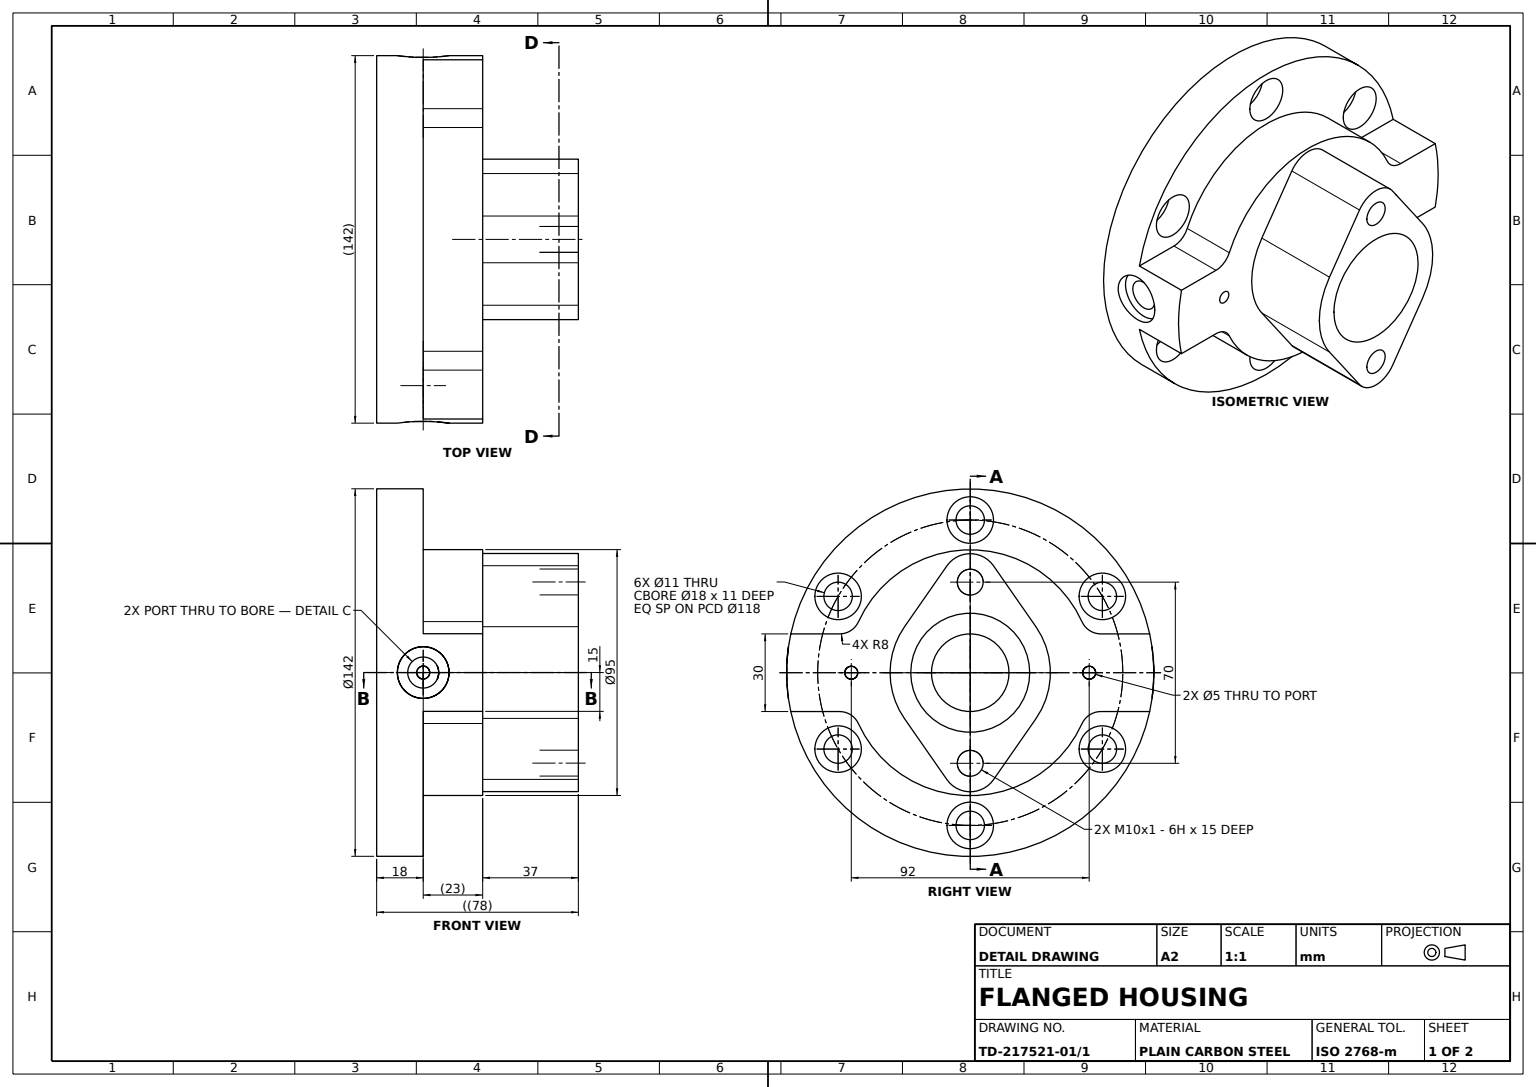
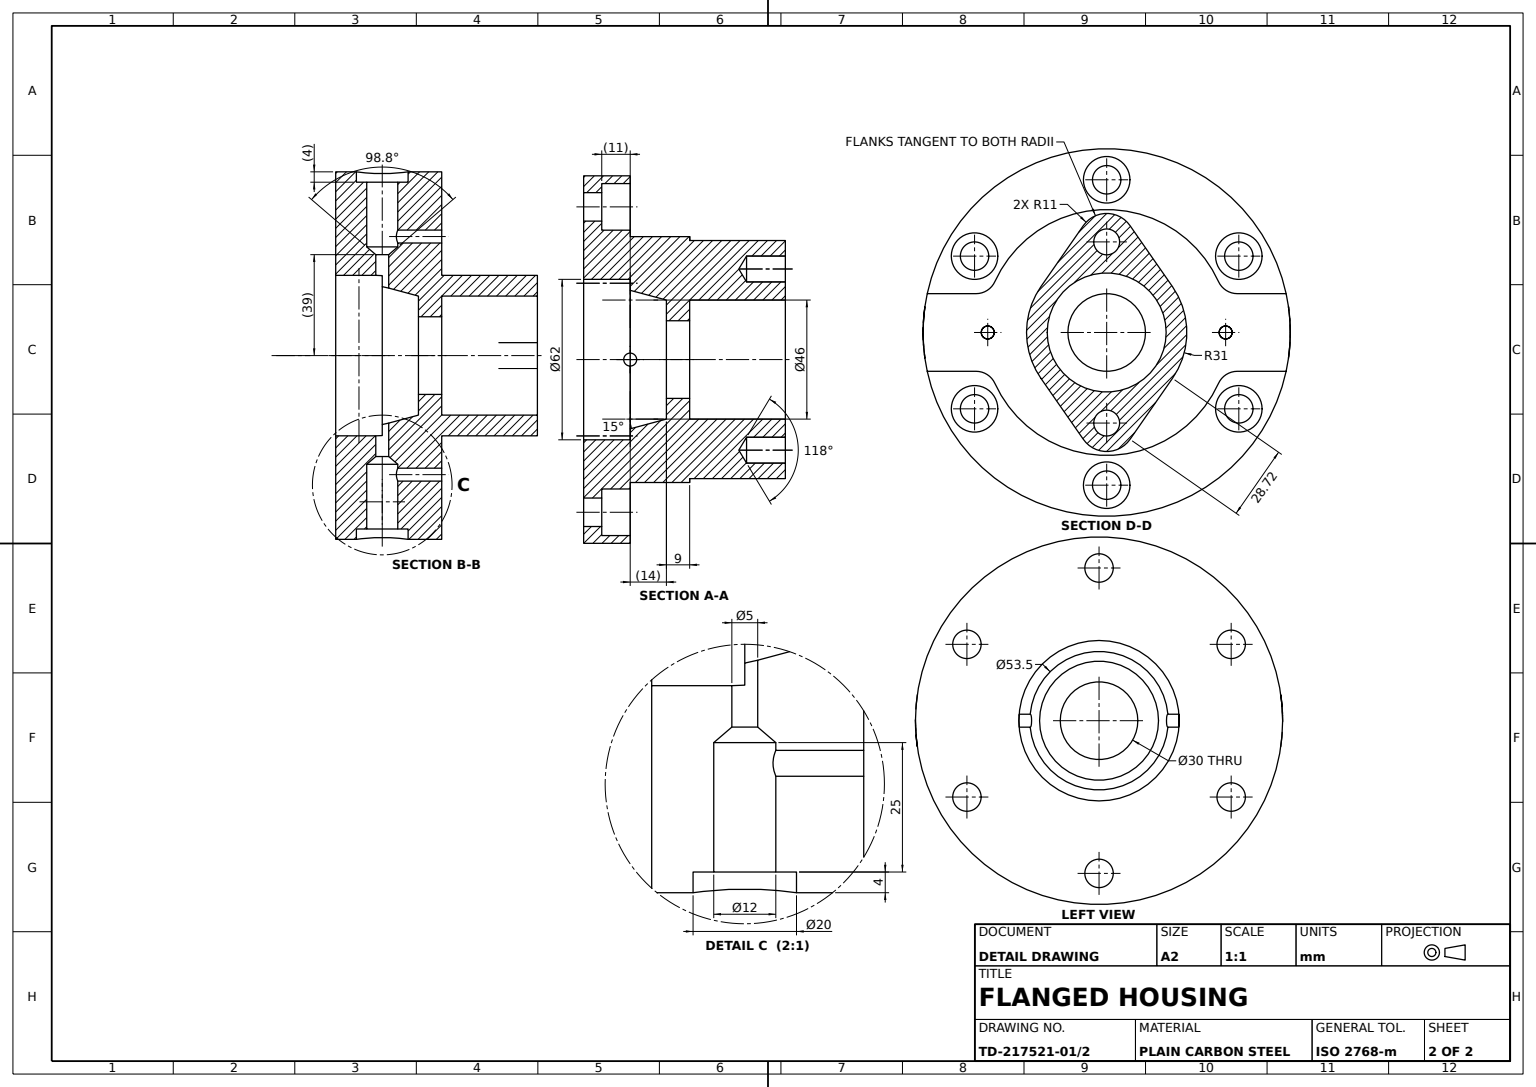
from build123d import *

# Parameters (mm, degrees)
BASE_FLANGE_SKETCH_R                   = 71
BASE_FLANGE_142_DEPTH                  = 18
MIDDLE_START                           = 23
MIDDLE_BOSS_DEPTH                      = 23
OVAL_FLANGE_SKETCH_R                   = 23
OVAL_TOP_FLANGE_DEPTH                  = 37
COUNTERBORED_BOLT_HOLE_M10_D           = 11
COUNTERBORED_BOLT_HOLE_M10_CBORE_D     = 18
COUNTERBORED_BOLT_HOLE_M10_CBORE_DEPTH = 11
BOLT_HOLE_PATTERN_6X_COUNT             = 6
CLEARANCE_HOLE_M5_D                    = 5
CLEARANCE_HOLE_M5_DEPTH                = 18
CLEARANCE_HOLE_M5_TIP                  = 1.502151548
TAPPED_HOLE_M10X1_0_D                  = 10
TAPPED_HOLE_M10X1_0_DEPTH              = 15
TAPPED_HOLE_M10X1_0_TIP                = 3.004303095


with BuildPart() as part:
    # Base Flange Sketch → Base Flange Ø142 (new body)
    with BuildSketch(Plane.XY):
        Circle(BASE_FLANGE_SKETCH_R)
    extrude(amount=BASE_FLANGE_142_DEPTH)

    # Middle Boss Sketch → Middle Boss (add)
    with BuildSketch(Plane(origin=(0, 0, 0), x_dir=(-1, 0, 0), z_dir=(0, 0, -1)).offset(MIDDLE_START)):
        with BuildLine():
            Line((50.50990002, 15), (69.397406292, 15))
            ThreePointArc((69.397406292, 15), (71, 0), (69.397406292, -15))
            Line((69.397406292, -15), (50.50990002, -15))
            ThreePointArc((50.50990002, -15), (46.181073535, -16.272350986), (43.229193711, -19.684684685))
            ThreePointArc((43.229193711, -19.684684685), (0, -47.5), (-43.229193711, -19.684684685))
            ThreePointArc((-43.229193711, -19.684684685), (-46.181073535, -16.272350986), (-50.50990002, -15))
            Line((-50.50990002, -15), (-69.397406292, -15))
            ThreePointArc((-69.397406292, -15), (-71, 0), (-69.397406292, 15))
            Line((-69.397406292, 15), (-50.50990002, 15))
            ThreePointArc((-50.50990002, 15), (-46.181073535, 16.272350986), (-43.229193711, 19.684684685))
            ThreePointArc((-43.229193711, 19.684684685), (0, 47.5), (43.229193711, 19.684684685))
            ThreePointArc((43.229193711, 19.684684685), (46.181073535, 16.272350986), (50.50990002, 15))
        make_face()
    extrude(amount=-MIDDLE_BOSS_DEPTH)

    # Oval Flange Sketch → Oval Top Flange (add)
    with BuildSketch(Plane(origin=(0, 0, -23), x_dir=(-1, 0, 0), z_dir=(0, 0, -1))):
        with BuildLine():
            Line((-9.027169873, 41.285714286), (-25.440206006, 17.714285714))
            ThreePointArc((-25.440206006, 17.714285714), (-31, 0), (-25.440206006, -17.714285714))
            Line((-25.440206006, -17.714285714), (-9.027169873, -41.285714286))
            ThreePointArc((-9.027169873, -41.285714286), (0, -46), (9.027169873, -41.285714286))
            Line((9.027169873, -41.285714286), (25.440206006, -17.714285714))
            ThreePointArc((25.440206006, -17.714285714), (31, 0), (25.440206006, 17.714285714))
            Line((25.440206006, 17.714285714), (9.027169873, 41.285714286))
            ThreePointArc((9.027169873, 41.285714286), (0, 46), (-9.027169873, 41.285714286))
        make_face()
        Circle(OVAL_FLANGE_SKETCH_R, mode=Mode.SUBTRACT)
    extrude(amount=OVAL_TOP_FLANGE_DEPTH)

    # Counterbored Bolt Hole M10 (through all)
    with Locations(Plane(origin=(0, 0, 0), x_dir=(-1, 0, 0), z_dir=(0, 0, -1))):
        with Locations((0, -59)):
            counterbored_bolt_hole_m10 = CounterBoreHole(COUNTERBORED_BOLT_HOLE_M10_D / 2, COUNTERBORED_BOLT_HOLE_M10_CBORE_D / 2, COUNTERBORED_BOLT_HOLE_M10_CBORE_DEPTH)

    # Bolt Hole Pattern 6x: Counterbored Bolt Hole M10 ×6 about axis
    bolt_hole_pattern_6x_axis = Axis((0, 0, 0), (0, 0, 1))
    for i in range(1, BOLT_HOLE_PATTERN_6X_COUNT):
        add(counterbored_bolt_hole_m10.rotate(bolt_hole_pattern_6x_axis, i * 360 / BOLT_HOLE_PATTERN_6X_COUNT), mode=Mode.SUBTRACT)

    # Central Bore Profile → Central Bore (revolve, cut)
    with BuildSketch(Plane(origin=(0, 0, 0), x_dir=(1, 0, 0), z_dir=(0, 1, 0)), mode=Mode.PRIVATE) as central_bore_sk:
        Polygon((0, 23), (0, -18), (31, -18), (31, 0), (26.751288694, 0), (23, 14), (15, 14), (15, 23), align=None)
    revolve(central_bore_sk.sketch.rotate(Axis((0, 0, -23), (0, 0, 1)), 180), axis=Axis((0, 0, -23), (0, 0, 1)), mode=Mode.SUBTRACT)

    # Side Port Profile → Side Port (revolve, cut)
    with BuildSketch(Plane(origin=(0, 0, 0), x_dir=(1, 0, 0), z_dir=(0, 1, 0))):
        Polygon((15.299257969, -2.5), (15.299257969, 0), (71, 0), (71, -10), (67, -10), (67, -6), (42, -6), (39, -2.5), align=None)
    side_port = revolve(axis=Axis((-79.296087495, 0, 0), (1, 0, 0)), mode=Mode.SUBTRACT)

    # Side Port Mirror: Side Port across plane
    add(side_port.mirror(Plane(origin=(0, 0, 0), x_dir=(0, 0, 1), z_dir=(1, 0, 0))), mode=Mode.SUBTRACT)

    # Clearance Hole M5
    with Locations(Plane(origin=(0, 0, -23), x_dir=(-1, 0, 0), z_dir=(0, 0, -1))):
        with Locations((-46, 0), (46, 0)):
            Hole(CLEARANCE_HOLE_M5_D / 2, depth=CLEARANCE_HOLE_M5_DEPTH)
            with Locations((0, 0, -(CLEARANCE_HOLE_M5_DEPTH + CLEARANCE_HOLE_M5_TIP / 2))):  # 118° drill point
                Cone(0, CLEARANCE_HOLE_M5_D / 2, CLEARANCE_HOLE_M5_TIP, mode=Mode.SUBTRACT)

    # Tapped Hole M10x1.0
    with Locations(Plane(origin=(0, 0, -60), x_dir=(-1, 0, 0), z_dir=(0, 0, -1))):
        with Locations((0, -35), (0, 35)):
            Hole(TAPPED_HOLE_M10X1_0_D / 2, depth=TAPPED_HOLE_M10X1_0_DEPTH)
            with Locations((0, 0, -(TAPPED_HOLE_M10X1_0_DEPTH + TAPPED_HOLE_M10X1_0_TIP / 2))):  # 118° drill point
                Cone(0, TAPPED_HOLE_M10X1_0_D / 2, TAPPED_HOLE_M10X1_0_TIP, mode=Mode.SUBTRACT)


solid = part.part
